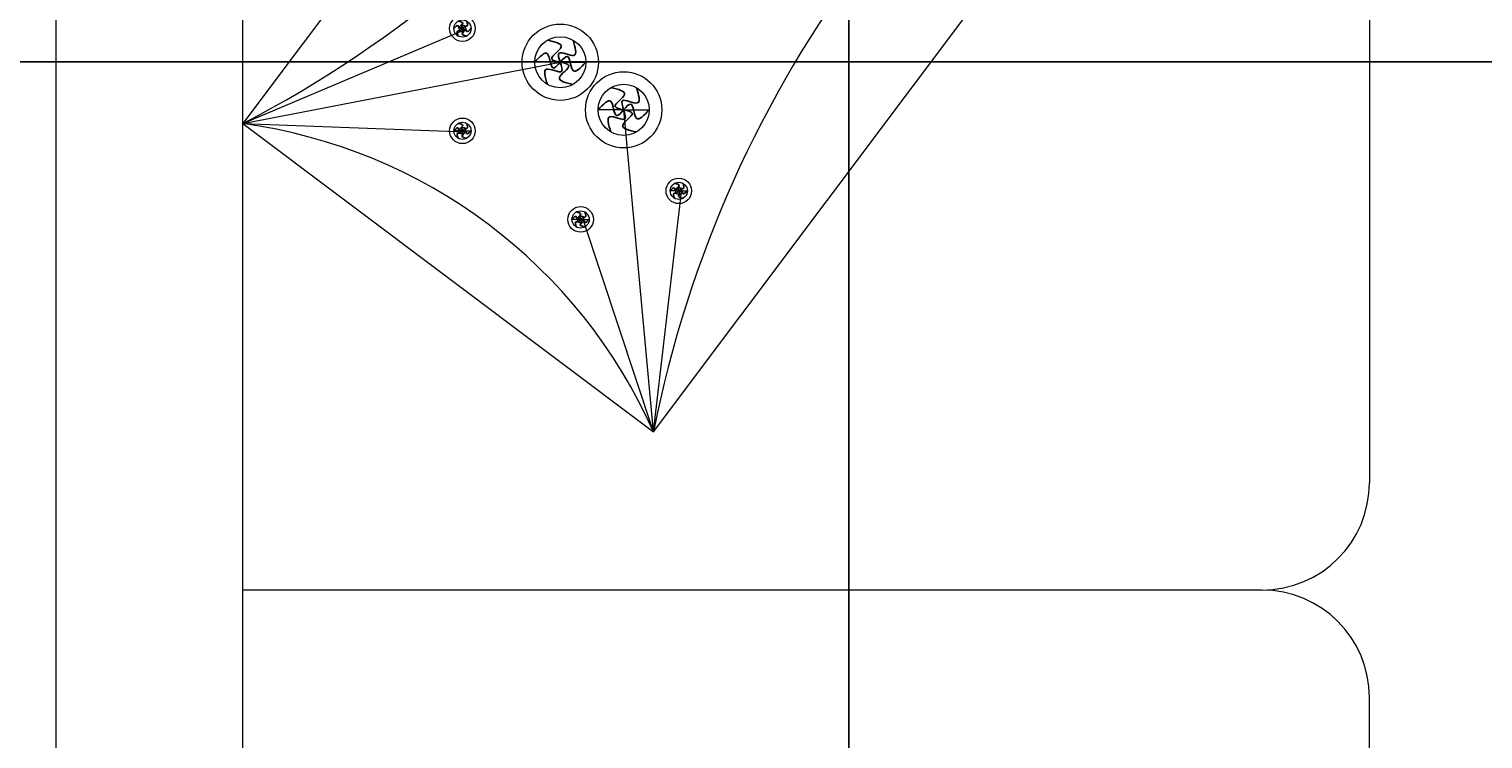
# Model space of a CAD drawing. Units: inches. Extents: x -61 to 1599, y -1316 to 257.
# Tile 26 of 204: x 388 to 416, y -886 to -873. Entities that reach past the tile are written whole.
import ezdxf

# ---------------------------------------------------------------- set-up
doc = ezdxf.new("R2010")
doc.units = ezdxf.units.IN
doc.header["$MEASUREMENT"] = 0
doc.layers.add('A-ANNO-DIMS', color=2, linetype='Continuous', lineweight=18)
doc.layers.add('FURNITURE', color=83, linetype='Continuous', lineweight=18)
doc.layers.add('FUR', color=83, linetype='Continuous')
doc.styles.get("Standard").update_dxf_attribs({"font": 'arial.ttf'})
doc.dimstyles.get("Standard").update_dxf_attribs({"dimtxt": 0.18, "dimasz": 0.18, "dimexe": 0.18, "dimexo": 0.0625, "dimgap": 0.09, "dimtad": 0, "dimtih": 1, "dimtoh": 1, "dimdec": 0, "dimzin": 0, "dimdsep": 46, "dimlunit": 3, "dimtxsty": 'Standard', "dimcen": 0.09, "dimadec": 0, "dimazin": 0, "dimtfac": 1, "dimtdec": 0, "dimtofl": 0, "dimtmove": 0, "dimatfit": 3, "dimfxl": 1, "dimtolj": 1, "dimtzin": 0, "dimarcsym": 0})

# ---------------------------------------------------------------- blocks, each defined once
blk = doc.blocks.new('*U186')
at = {"layer": 'FUR'}
blk.add_open_spline([(0.005, 0.08), (-0.03, 0.048), (-0.098, -0.015), (0.075, -0.018), (0.024, -0.063), (0.005, -0.08)], degree=3, knots=[0, 0, 0, 0, 0.0954578, 0.1898773, 0.2470677, 0.2470677, 0.2470677, 0.2470677], dxfattribs=at)
blk = doc.blocks.new('*U187')
at = {"layer": 'FUR', "transparency": 16777216}
for p, rotation in [((222.173, -79.977), 60), ((222.178, -80.056), 120), ((222.25, -80.092), 180), ((222.312, -79.968), 300), ((222.317, -80.048), 240)]:
    blk.add_blockref('*U186', p, dxfattribs=dict(at, rotation=rotation))
blk.add_blockref('*U186', (222.24, -79.932), dxfattribs=at)
blk = doc.blocks.new('*U198')
at = {"layer": 'FUR'}
blk.add_open_spline([(0.005, 0.08), (-0.03, 0.048), (-0.098, -0.015), (0.075, -0.018), (0.024, -0.063), (0.005, -0.08)], degree=3, knots=[0, 0, 0, 0, 0.0954578, 0.1898773, 0.2470677, 0.2470677, 0.2470677, 0.2470677], dxfattribs=at)
blk = doc.blocks.new('*U199')
at = {"layer": 'FUR', "transparency": 16777216}
for p, rotation in [((222.173, -79.977), 60), ((222.178, -80.056), 120), ((222.25, -80.092), 180), ((222.312, -79.968), 300), ((222.317, -80.048), 240)]:
    blk.add_blockref('*U198', p, dxfattribs=dict(at, rotation=rotation))
blk.add_blockref('*U198', (222.24, -79.932), dxfattribs=at)
blk = doc.blocks.new('*U210')
at = {"layer": 'FUR'}
blk.add_open_spline([(0.015, 0.238), (-0.088, 0.143), (-0.292, -0.045), (0.224, -0.053), (0.072, -0.187), (0.015, -0.238)], degree=3, knots=[0, 0, 0, 0, 0.2846533, 0.5662105, 0.736751, 0.736751, 0.736751, 0.736751], dxfattribs=at)
blk = doc.blocks.new('*U185')
at = {"layer": 'FUR', "transparency": 16777216}
blk.add_blockref('*U210', (662.716, -238.357), dxfattribs=at)
for p, rotation in [((662.517, -238.489), 60), ((662.929, -238.463), 300), ((662.531, -238.727), 120), ((662.745, -238.833), 180), ((662.944, -238.702), 240)]:
    blk.add_blockref('*U210', p, dxfattribs=dict(at, rotation=rotation))
blk = doc.blocks.new('*U200')
at = {"layer": 'FUR'}
blk.add_open_spline([(0.005, 0.08), (-0.03, 0.048), (-0.098, -0.015), (0.075, -0.018), (0.024, -0.063), (0.005, -0.08)], degree=3, knots=[0, 0, 0, 0, 0.0954578, 0.1898773, 0.2470677, 0.2470677, 0.2470677, 0.2470677], dxfattribs=at)
blk = doc.blocks.new('*U201')
at = {"layer": 'FUR', "transparency": 16777216}
for p, rotation in [((222.173, -79.977), 60), ((222.178, -80.056), 120), ((222.25, -80.092), 180), ((222.312, -79.968), 300), ((222.317, -80.048), 240)]:
    blk.add_blockref('*U200', p, dxfattribs=dict(at, rotation=rotation))
blk.add_blockref('*U200', (222.24, -79.932), dxfattribs=at)
blk = doc.blocks.new('*U194')
at = {"layer": 'FUR'}
blk.add_open_spline([(0.015, 0.238), (-0.088, 0.143), (-0.292, -0.045), (0.224, -0.053), (0.072, -0.187), (0.015, -0.238)], degree=3, knots=[0, 0, 0, 0, 0.2846533, 0.5662105, 0.736751, 0.736751, 0.736751, 0.736751], dxfattribs=at)
blk = doc.blocks.new('*U195')
at = {"layer": 'FUR', "transparency": 16777216}
blk.add_blockref('*U194', (662.716, -238.357), dxfattribs=at)
for p, rotation in [((662.517, -238.489), 60), ((662.929, -238.463), 300), ((662.531, -238.727), 120), ((662.745, -238.833), 180), ((662.944, -238.702), 240)]:
    blk.add_blockref('*U194', p, dxfattribs=dict(at, rotation=rotation))
blk = doc.blocks.new('*U202')
at = {"layer": 'FUR'}
blk.add_open_spline([(0.005, 0.08), (-0.03, 0.048), (-0.098, -0.015), (0.075, -0.018), (0.024, -0.063), (0.005, -0.08)], degree=3, knots=[0, 0, 0, 0, 0.0954578, 0.1898773, 0.2470677, 0.2470677, 0.2470677, 0.2470677], dxfattribs=at)
blk = doc.blocks.new('*U203')
at = {"layer": 'FUR', "transparency": 16777216}
for p, rotation in [((222.173, -79.977), 60), ((222.178, -80.056), 120), ((222.25, -80.092), 180), ((222.312, -79.968), 300), ((222.317, -80.048), 240)]:
    blk.add_blockref('*U202', p, dxfattribs=dict(at, rotation=rotation))
blk.add_blockref('*U202', (222.24, -79.932), dxfattribs=at)
blk = doc.blocks.new('SOFA-LOVESEAT')
for p, q in [((3.47, 8), (3.47, 52)), ((24.442, 52), (24.442, 32)), ((3.47, 38.686), (7.612, 40.436)), ((3.47, 38.686), (9.381, 39.828)), ((9.381, 39.828), (8.904, 39.828)), ((9.381, 39.828), (9.857, 39.828)), ((10.561, 38.942), (10.084, 38.942)), ((11.116, 32.948), (10.561, 38.942)), ((10.561, 38.942), (11.037, 38.942)), ((3.47, 38.686), (7.612, 38.532)), ((7.56, 38.551), (7.4, 38.551)), ((7.56, 38.551), (7.719, 38.551)), ((11.116, 32.948), (11.639, 37.414)), ((11.587, 37.433), (11.427, 37.433)), ((11.587, 37.433), (11.747, 37.433)), ((9.759, 36.901), (9.599, 36.901)), ((9.759, 36.901), (9.918, 36.901)), ((11.116, 32.948), (9.811, 36.882)), ((22.442, 30), (3.47, 30)), ((22.442, 30), (22.442, 30)), ((24.442, 8), (24.442, 28))]:
    blk.add_line(p, q)
blk.add_lwpolyline([(26, 6), (26, 2, -0.414214), (24, 0), (2, 0, -0.414214), (0, 2), (0, 58, -0.414213), (2, 60), (24, 60, -0.414214), (26, 58), (26, 54)], format="xyb")
blk.add_lwpolyline([(11.116, 32.948), (22.422, 48.013), (14.776, 53.751), (3.47, 38.686)], close=True)
for centre, radius in [((7.56, 40.455), 0.238), ((7.56, 40.455), 0.16), ((9.381, 39.828), 0.71), ((9.381, 39.828), 0.476), ((10.561, 38.942), 0.71), ((10.561, 38.942), 0.476), ((7.56, 38.551), 0.238), ((7.56, 38.551), 0.16), ((11.587, 37.433), 0.238), ((11.587, 37.433), 0.16), ((9.759, 36.901), 0.238), ((9.759, 36.901), 0.16)]:
    blk.add_circle(centre, radius)
for centre, radius, start, end in [((-6.541, 57.974), 21.731, 297.4317, 348.7956), ((32.433, 28.726), 21.731, 117.4317, 168.7956), ((2.147, 28.96), 9.816, 23.9742, 82.253), ((22.442, 32), 2, 270, 0), ((22.442, 28), 2, 0, 90)]:
    blk.add_arc(centre, radius, start, end)
at = {"xscale": -1, "rotation": 90.00003000000098}
for name, p in [('*U187', (-72.453, 262.7)), ('*U185', (-229.215, 702.558)), ('*U195', (-228.035, 701.672)), ('*U199', (-72.453, 260.796)), ('*U203', (-68.426, 259.678)), ('*U201', (-70.254, 259.146))]:
    blk.add_blockref(name, p, dxfattribs=at)
blk = doc.blocks.new('*D696')
at = {"layer": 'A-ANNO-DIMS', "color": 0, "lineweight": -2, "transparency": 16777216}
for p, q in [((690.64, -873.169), (-61.077, -873.169)), ((-60.897, -873.349), (-60.897, -1025.799)), ((-60.897, -1178.613), (-60.897, -1026.163)), ((690.64, -1178.793), (-61.077, -1178.793))]:
    blk.add_line(p, q, dxfattribs=at)
at = {"layer": 'A-ANNO-DIMS', "color": 0, "transparency": 16777216}
for points in [[(-60.927, -873.349), (-60.867, -873.349), (-60.897, -873.169)], [(-60.927, -1178.613), (-60.867, -1178.613), (-60.897, -1178.793)]]:
    blk.add_solid(points, dxfattribs=at)
at = {"layer": 'DEFPOINTS', "color": 0, "transparency": 16777216}
for p in [(-60.897, -873.169), (690.703, -873.169), (690.703, -1178.793)]:
    blk.add_point(p, dxfattribs=at)
at = {"layer": 'A-ANNO-DIMS', "color": 0, "transparency": 16777216, "insert": (-60.897, -1025.981), "char_height": 0.18, "attachment_point": 5}
blk.add_mtext('\\A1;305.6', dxfattribs=at)
blk = doc.blocks.new('*D710')
at = {"layer": 'A-ANNO-DIMS', "color": 0, "lineweight": -2, "transparency": 16777216}
for p, q in [((319.703, -465.385), (319.703, -1315.725)), ((403.703, -465.385), (403.703, -1315.725)), ((319.883, -1315.545), (361.484, -1315.545)), ((403.523, -1315.545), (361.921, -1315.545))]:
    blk.add_line(p, q, dxfattribs=at)
at = {"layer": 'A-ANNO-DIMS', "color": 0, "transparency": 16777216}
for points in [[(319.883, -1315.515), (319.883, -1315.575), (319.703, -1315.545)], [(403.523, -1315.515), (403.523, -1315.575), (403.703, -1315.545)]]:
    blk.add_solid(points, dxfattribs=at)
at = {"layer": 'DEFPOINTS', "color": 0, "transparency": 16777216}
for p in [(319.703, -465.323), (403.703, -465.323), (403.703, -1315.545)]:
    blk.add_point(p, dxfattribs=at)
at = {"layer": 'A-ANNO-DIMS', "color": 0, "transparency": 16777216, "insert": (361.703, -1315.545), "char_height": 0.18, "attachment_point": 5}
blk.add_mtext('\\A1;84', dxfattribs=at)

msp = doc.modelspace()

# ---------------------------------------------------------------- block references
at = {"layer": 'FURNITURE'}
msp.add_blockref('SOFA-LOVESEAT', (388.9518, -913.0047), dxfattribs=at)

# ---------------------------------------------------------------- dimensions: what is measured, and where the dimension line sits
at = {"layer": 'A-ANNO-DIMS'}
dim = msp.add_linear_dim(base=(403.7028, -1315.5446), p1=(319.7028, -465.3229), p2=(403.7028, -465.3229), dimstyle='Standard', override={"dimdec": 0, "dimlfac": 1, "dimrnd": 0, "dimzin": 0, "dimdsep": 46, "dimlunit": 2}, dxfattribs=at)
dim.commit()
dim.dimension.update_dxf_attribs({"geometry": '*D710', "text_midpoint": (361.7028, -1315.5446)})
dim = msp.add_linear_dim(base=(-60.8972, -873.169), p1=(690.7028, -1178.7933), p2=(690.7028, -873.169), angle=90, dimstyle='Standard', override={"dimdec": 1, "dimlfac": 1, "dimrnd": 0, "dimzin": 0, "dimdsep": 46, "dimlunit": 2}, dxfattribs=at)
dim.commit()
dim.dimension.update_dxf_attribs({"geometry": '*D696', "text_midpoint": (-60.8972, -1025.9812)})

doc.saveas('drawing.dxf')
